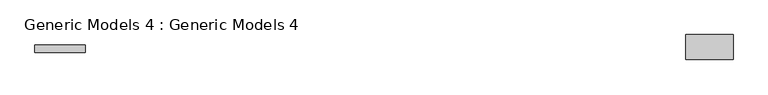
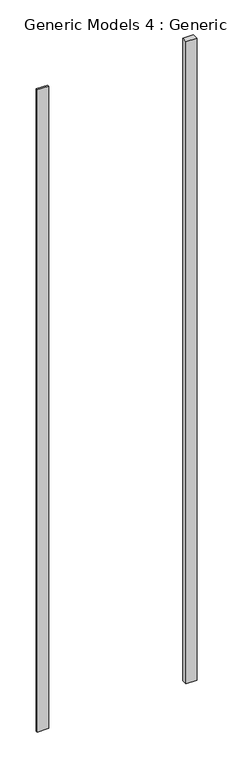
"""IFC4 building model written with IfcOpenShell, lengths in millimetres: proxy geometry, Generic Models 4 : Generic Models 4."""

from ifc_helpers import new_model, si_unit, origin, origin_with_axes, place, context, project, spatial, polyline, outline, extrude, source, transform, mapped, element, save


def generic_models_4_generic_models_4_c09d9ab6(model_context):
    return source(origin(), model_context, "Body", "SweptSolid", [
        extrude(outline(polyline([(-377.8108866, -2898.9540153), (-377.8108866, -2867.8939202), (-174.6108866, -2867.8939202), (-174.6108866, -2898.9540153), (-377.8108866, -2898.9540153)])), origin_with_axes(), (0.0, 0.0, 1.0), 12087.9214585),
        extrude(outline(polyline([(2261.7907316, -2927.0989911), (2261.7907316, -2826.2789605), (2454.2891134, -2826.2789605), (2454.2891134, -2927.0989911), (2261.7907316, -2927.0989911)])), origin_with_axes(), (0.0, 0.0, 1.0), 12087.9214585),
    ])


if __name__ == "__main__":
    model = new_model("IFC4")
    model_context = context("Model", 3, world=origin())
    ifc_project = project(units=[si_unit("LENGTHUNIT", "METRE", prefix="MILLI")], contexts=[model_context])
    site = spatial("IfcSite", under=ifc_project)
    building = spatial("IfcBuilding", under=site)
    placement = place(None, origin())
    generic_models_4_generic_models_4_shape = generic_models_4_generic_models_4_c09d9ab6(model_context)
    element("IfcBuildingElementProxy", 1, Name="Generic Models 4 : Generic Models 4", ObjectType="Generic Models 4 : Generic Models 4", at=placement, inside=building, context=model_context, shape_type="MappedRepresentation", body=[
        mapped(generic_models_4_generic_models_4_shape, transform((0.0, 0.0, 0.0), x_axis=(1.0, 0.0, 0.0), y_axis=(0.0, 1.0, 0.0), z_axis=(0.0, 0.0, 1.0))),
    ])
    save(model, "model.ifc")

# Revit data of these elements
# Element 1 (IfcBuildingElementProxy, "Generic Models 4 : Generic Models 4")
#   Materials on its faces: "Oak Flooring", "Window Frame"
# Materials
#   "Oak Flooring": class "Wood", colour RGB 216 169 114, transparency 0, Description = "Quercus Rubra", Cost = 0
#   "Window Frame": colour RGB 249 249 249, transparency 0
